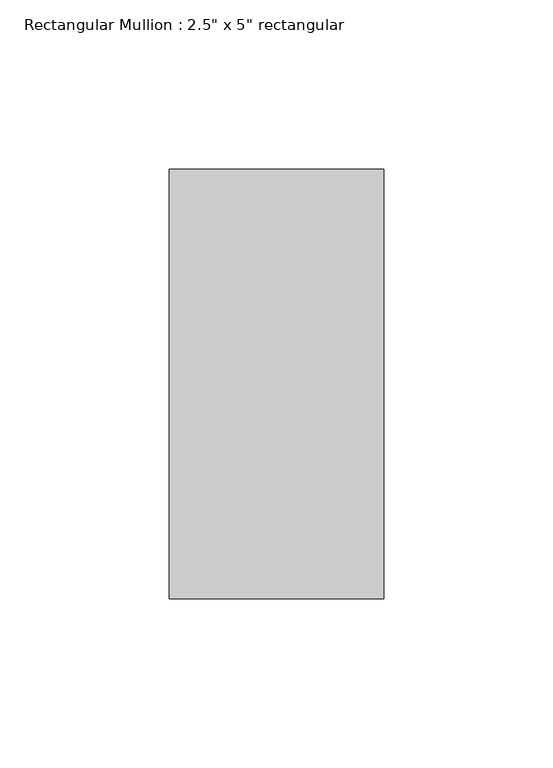
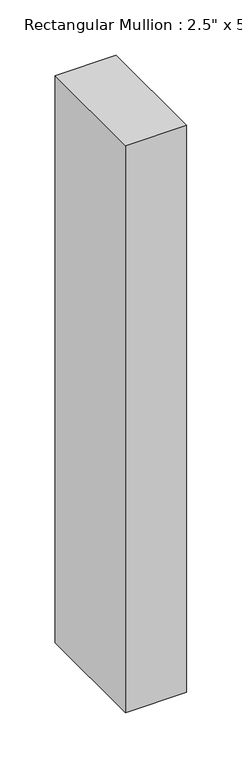
"""IFC4 building model written with IfcOpenShell, lengths in millimetres: member geometry."""

from ifc_helpers import new_model, si_unit, frame, origin, place, context, project, spatial, polyline, outline, extrude, source, transform, mapped, element, save


def member_0bb20091(model_context):
    return source(origin(), model_context, "Body", "SweptSolid", [
        extrude(outline(polyline([(0.0, 63.5), (0.0, -63.5), (-63.5, -63.5), (-63.5, 63.5), (0.0, 63.5)])), frame((0.0, 0.0, -624.6708479), z_axis=(0.0, 0.0, 1.0), x_axis=(1.0, 0.0, 0.0)), (0.0, 0.0, 1.0), 624.6708479),
    ])


if __name__ == "__main__":
    model = new_model("IFC4")
    model_context = context("Model", 3, world=origin())
    ifc_project = project(units=[si_unit("LENGTHUNIT", "METRE", prefix="MILLI")], contexts=[model_context])
    site = spatial("IfcSite", under=ifc_project)
    building = spatial("IfcBuilding", under=site)
    placement = place(None, origin())
    member_shape = member_0bb20091(model_context)
    element("IfcMember", 1, ObjectType="Rectangular Mullion : 2.5\" x 5\" rectangular", at=placement, inside=building, context=model_context, shape_type="MappedRepresentation", body=[
        mapped(member_shape, transform((0.0, 0.0, 0.0), x_axis=(1.0, 0.0, 0.0), y_axis=(0.0, 1.0, 0.0), z_axis=(0.0, 0.0, 1.0))),
    ])
    save(model, "model.ifc")

# Revit data of these elements
# Type "Rectangular Mullion : 2.5\" x 5\" rectangular"
#   built-in parameter 1007304 = 0.416667 (stored number, unit not read)
#   built-in parameter 1007301 = 0.104167 (stored number, unit not read)
#   built-in parameter 1007300 = 0.104167 (stored number, unit not read)
# Element 1 (IfcMember, "Rectangular Mullion : 2.5\" x 5\" rectangular")
#   Materials on its faces: "Aluminum"
# Materials
#   "Aluminum": class "Metal", colour RGB 247 247 247, transparency 0, Description = "Aluminum 6061", Cost = 0
